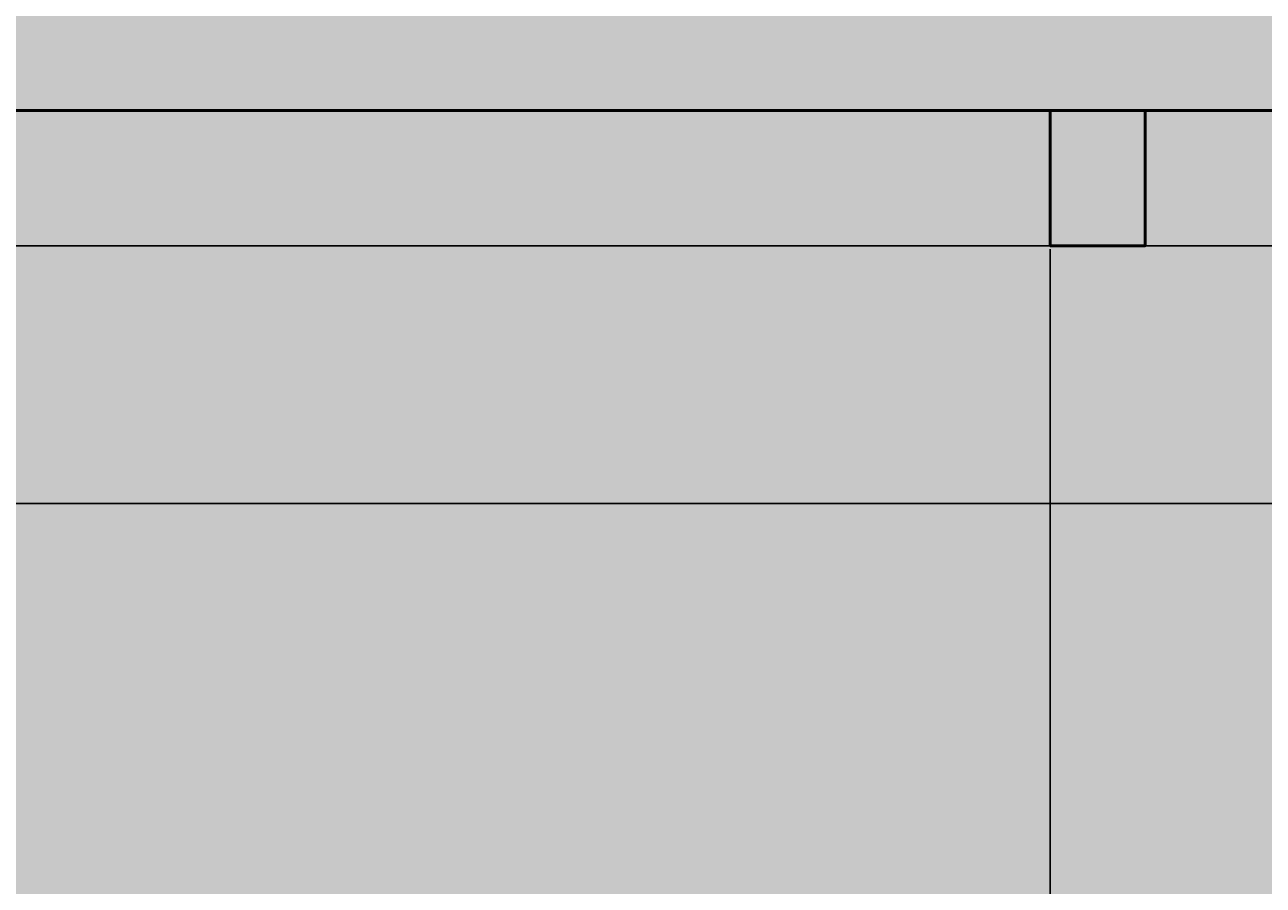
# Model space of a CAD drawing. Units: inches. Extents: x -12 to 334, y -10 to 186.
# Tile 41 of 77: x 152 to 175, y 49 to 65. Entities that reach past the tile are written whole.
import ezdxf

# ---------------------------------------------------------------- set-up
doc = ezdxf.new("R2010")
doc.units = ezdxf.units.IN
doc.header["$MEASUREMENT"] = 0
for name, color, linetype, lineweight in [('M-DIMS', 2, 'Continuous', 18), ('M-EQPM', 7, 'Continuous', 50), ('M-EQPM-PATT', 8, 'Continuous', 18)]:
    doc.layers.add(name, color=color, linetype=linetype, lineweight=lineweight)
doc.styles.get("Standard").update_dxf_attribs({"font": 'arial.ttf'})
doc.dimstyles.get("Standard").update_dxf_attribs({"dimtxt": 0.18, "dimasz": 0.18, "dimexe": 0.18, "dimexo": 0.0625, "dimgap": 0.09, "dimtad": 0, "dimtih": 1, "dimtoh": 1, "dimdec": 4, "dimzin": 0, "dimdsep": 46, "dimtxsty": 'Standard', "dimcen": 0.09, "dimadec": 0, "dimazin": 0, "dimtfac": 1, "dimtdec": 4, "dimtofl": 0, "dimtmove": 0, "dimatfit": 3, "dimfxl": 1, "dimtolj": 1, "dimtzin": 0, "dimarcsym": 0})

# ---------------------------------------------------------------- blocks, each defined once
blk = doc.blocks.new('*D1')
at = {"layer": 'Defpoints', "color": 0, "transparency": 16777216}
for p in [(281.426, 91.899), (3.376, 80.692), (281.426, 14.304)]:
    blk.add_point(p, dxfattribs=at)
at = {"layer": 'M-DIMS', "color": 0, "lineweight": -2, "transparency": 16777216}
for p, q in [((281.426, 91.836), (281.426, 14.124)), ((3.376, 80.629), (3.376, 14.124)), ((3.556, 14.304), (141.935, 14.304)), ((281.246, 14.304), (142.867, 14.304))]:
    blk.add_line(p, q, dxfattribs=at)
at = {"layer": 'M-DIMS', "color": 0, "transparency": 16777216}
for points in [[(3.556, 14.334), (3.556, 14.274), (3.376, 14.304)], [(281.246, 14.334), (281.246, 14.274), (281.426, 14.304)]]:
    blk.add_solid(points, dxfattribs=at)
at = {"layer": 'M-DIMS', "color": 0, "transparency": 16777216, "insert": (142.401, 14.304), "char_height": 0.18, "attachment_point": 5}
blk.add_mtext('\\A1;278.05', dxfattribs=at)
blk = doc.blocks.new('*D17')
at = {"layer": 'Defpoints', "color": 0, "transparency": 16777216}
for p in [(106.177, 102.896), (105.892, 56.321), (295.976, 56.321)]:
    blk.add_point(p, dxfattribs=at)
at = {"layer": 'M-DIMS', "color": 0, "lineweight": -2, "transparency": 16777216}
for p, q in [((106.24, 102.896), (296.156, 102.896)), ((295.976, 102.716), (295.976, 79.79)), ((295.976, 56.501), (295.976, 79.426)), ((105.954, 56.321), (296.156, 56.321))]:
    blk.add_line(p, q, dxfattribs=at)
at = {"layer": 'M-DIMS', "color": 0, "transparency": 16777216}
for points in [[(295.946, 102.716), (296.006, 102.716), (295.976, 102.896)], [(295.946, 56.501), (296.006, 56.501), (295.976, 56.321)]]:
    blk.add_solid(points, dxfattribs=at)
at = {"layer": 'M-DIMS', "color": 0, "transparency": 16777216, "insert": (295.976, 79.608), "char_height": 0.18, "attachment_point": 5}
blk.add_mtext('\\A1;46.575', dxfattribs=at)
blk = doc.blocks.new('*D31')
at = {"layer": 'Defpoints', "color": 0, "transparency": 16777216}
for p in [(129.093, 61.105), (170.908, 61.105), (170.908, 14.304)]:
    blk.add_point(p, dxfattribs=at)
at = {"layer": 'M-DIMS', "color": 0, "lineweight": -2, "transparency": 16777216}
for p, q in [((129.093, 61.042), (129.093, 14.124)), ((170.908, 61.042), (170.908, 14.124)), ((129.273, 14.304), (149.532, 14.304)), ((170.728, 14.304), (150.468, 14.304))]:
    blk.add_line(p, q, dxfattribs=at)
at = {"layer": 'M-DIMS', "color": 0, "transparency": 16777216}
for points in [[(129.273, 14.334), (129.273, 14.274), (129.093, 14.304)], [(170.728, 14.334), (170.728, 14.274), (170.908, 14.304)]]:
    blk.add_solid(points, dxfattribs=at)
at = {"layer": 'M-DIMS', "color": 0, "transparency": 16777216, "insert": (150, 14.304), "char_height": 0.18, "attachment_point": 5}
blk.add_mtext('\\A1;41.815', dxfattribs=at)
blk = doc.blocks.new('*D32')
at = {"layer": 'Defpoints', "color": 0, "transparency": 16777216}
for p in [(170.908, 61.105), (216.428, 61.105), (216.428, 14.304)]:
    blk.add_point(p, dxfattribs=at)
at = {"layer": 'M-DIMS', "color": 0, "lineweight": -2, "transparency": 16777216}
for p, q in [((170.908, 61.042), (170.908, 14.124)), ((216.428, 61.042), (216.428, 14.124)), ((171.088, 14.304), (193.271, 14.304)), ((216.248, 14.304), (194.064, 14.304))]:
    blk.add_line(p, q, dxfattribs=at)
at = {"layer": 'M-DIMS', "color": 0, "transparency": 16777216}
for points in [[(171.088, 14.334), (171.088, 14.274), (170.908, 14.304)], [(216.248, 14.334), (216.248, 14.274), (216.428, 14.304)]]:
    blk.add_solid(points, dxfattribs=at)
at = {"layer": 'M-DIMS', "color": 0, "transparency": 16777216, "insert": (193.668, 14.304), "char_height": 0.18, "attachment_point": 5}
blk.add_mtext('\\A1;45.52', dxfattribs=at)
blk = doc.blocks.new('*D35')
at = {"layer": 'Defpoints', "color": 0, "transparency": 16777216}
for p in [(216.428, 98.108), (-11.174, 61.105), (216.428, 61.105)]:
    blk.add_point(p, dxfattribs=at)
at = {"layer": 'M-DIMS', "color": 0, "lineweight": -2, "transparency": 16777216}
for p, q in [((216.365, 98.108), (-11.354, 98.108)), ((-11.174, 97.928), (-11.174, 79.788)), ((-11.174, 61.285), (-11.174, 79.424)), ((216.365, 61.105), (-11.354, 61.105))]:
    blk.add_line(p, q, dxfattribs=at)
at = {"layer": 'M-DIMS', "color": 0, "transparency": 16777216}
for points in [[(-11.204, 97.928), (-11.144, 97.928), (-11.174, 98.108)], [(-11.204, 61.285), (-11.144, 61.285), (-11.174, 61.105)]]:
    blk.add_solid(points, dxfattribs=at)
at = {"layer": 'M-DIMS', "color": 0, "transparency": 16777216, "insert": (-11.174, 79.606), "char_height": 0.18, "attachment_point": 5}
blk.add_mtext('\\A1;37', dxfattribs=at)
blk = doc.blocks.new('*D39')
at = {"layer": 'Defpoints', "color": 0, "transparency": 16777216}
for p in [(279.726, 80.692), (-11.174, 45.854), (269.381, 45.854)]:
    blk.add_point(p, dxfattribs=at)
at = {"layer": 'M-DIMS', "color": 0, "lineweight": -2, "transparency": 16777216}
for p, q in [((279.664, 80.692), (-11.354, 80.692)), ((-11.174, 80.512), (-11.174, 63.455)), ((-11.174, 46.034), (-11.174, 63.091)), ((269.318, 45.854), (-11.354, 45.854))]:
    blk.add_line(p, q, dxfattribs=at)
at = {"layer": 'M-DIMS', "color": 0, "transparency": 16777216}
for points in [[(-11.204, 80.512), (-11.144, 80.512), (-11.174, 80.692)], [(-11.204, 46.034), (-11.144, 46.034), (-11.174, 45.854)]]:
    blk.add_solid(points, dxfattribs=at)
at = {"layer": 'M-DIMS', "color": 0, "transparency": 16777216, "insert": (-11.174, 63.273), "char_height": 0.18, "attachment_point": 5}
blk.add_mtext('\\A1;34.84', dxfattribs=at)

msp = doc.modelspace()

# ---------------------------------------------------------------- hatches: boundary and pattern name
at = {"layer": 'M-EQPM-PATT'}
h = msp.add_hatch(color=256, dxfattribs=at)
h.set_gradient(color1=(205, 32, 39), color2=(205, 32, 39), tint=1)
h.paths.add_polyline_path([(64.5, 80.754), (64.5, 89.8963), (226.6083, 89.8963, -1), (226.6083, 69.6117), (64.5, 69.6117), (64.5, 78.754), (4.4744, 78.754, 0.384914), (23.5807, 61.4872), (37.1002, 61.4872), (37.1002, 33.6752), (53.1002, 33.6752), (53.1002, 61.4872), (64.5, 61.4872), (64.5, 63.6117), (226.6083, 63.6117, 1), (226.6083, 95.8963), (64.5, 95.8963), (64.5, 99.8958), (53.1002, 99.8958), (53.1002, 127.7078), (37.1002, 127.7078), (37.1002, 99.8958), (23.5807, 99.8958, 0.4132606), (4.3766, 80.754)])
h.paths.add_polyline_path([(64.5, 91.8963), (64.5, 93.8963), (226.6083, 93.8963, -1), (226.6083, 65.6117), (64.5, 65.6117), (64.5, 67.6117), (226.6083, 67.6117, 1), (226.6083, 91.8963)], flags=16)
h = msp.add_hatch(color=256, dxfattribs=at)
h.set_gradient(color1=(99, 100, 102), color2=(99, 100, 102), tint=1)
h.paths.add_polyline_path([(72.9244, 95.8963), (75.9244, 95.8963), (75.9244, 109.0583), (72.9244, 109.0583)])
h.paths.add_polyline_path([(72.9244, 50.4497), (75.9244, 50.4497), (75.9244, 63.6117), (72.9244, 63.6117)])
h.paths.add_polyline_path([(75.9244, 91.8963), (75.9244, 93.8963), (72.9244, 93.8963), (72.9244, 91.8963)])
h.paths.add_polyline_path([(75.9244, 65.6117), (75.9244, 67.6117), (72.9244, 67.6117), (72.9244, 65.6117)])
h.paths.add_polyline_path([(129.093, 69.6117), (130.8573, 69.6117), (130.8573, 89.8963), (129.093, 89.8963)])
h.paths.add_polyline_path([(129.093, 98.1081), (129.093, 95.8963), (130.8573, 95.8963), (130.8573, 98.1081)])
h.paths.add_polyline_path([(130.8573, 61.1045), (130.8573, 63.6117), (129.093, 63.6117), (129.093, 61.1045)])
h.paths.add_polyline_path([(170.9079, 69.6117), (172.6722, 69.6117), (172.6722, 89.8963), (170.9079, 89.8963)])
h.paths.add_polyline_path([(172.6722, 95.8963), (172.6722, 98.1081), (170.9079, 98.1081), (170.9079, 95.8963)])
h.paths.add_polyline_path([(170.9079, 61.1045), (172.6722, 61.1045), (172.6722, 63.6117), (170.9079, 63.6117)])
h.paths.add_polyline_path([(218.1922, 63.6117), (216.4278, 63.6117), (216.4278, 61.1045), (218.1922, 61.1045)])
h.paths.add_polyline_path([(216.4278, 69.6117), (218.1922, 69.6117), (218.1922, 89.8963), (216.4278, 89.8963)])
h.paths.add_polyline_path([(216.4278, 95.8963), (218.1922, 95.8963), (218.1922, 98.1081), (216.4278, 98.1081)])
h = msp.add_hatch(color=256, dxfattribs=at)
h.set_gradient(color1=(94, 103, 175), color2=(94, 103, 175), tint=1)
h.paths.add_polyline_path([(129.093, 89.8963), (86.8879, 89.8963), (86.8879, 69.6117), (129.093, 69.6117)], flags=17)
h.paths.add_polyline_path([(170.9079, 89.8963), (130.8573, 89.8963), (130.8573, 69.6117), (170.9079, 69.6117)], flags=17)
h.paths.add_polyline_path([(216.4278, 89.8963), (172.6722, 89.8963), (172.6722, 69.6117), (216.4278, 69.6117)], flags=17)
h.paths.add_polyline_path([(245.9354, 82.6969), (247.9354, 82.6969), (247.9354, 46.8541), (268.3808, 46.8541, 0.0998398), (279.7263, 80.6915), (251.9801, 80.6915, 0.4142136), (231.7758, 100.8958), (84.7229, 100.8958), (84.7229, 109.0583), (83.7229, 109.0583), (83.7229, 95.8963), (129.093, 95.8963), (129.093, 98.1081), (130.8573, 98.1081), (130.8573, 95.8963), (170.9079, 95.8963), (170.9079, 98.1081), (172.6722, 98.1081), (172.6722, 95.8963), (216.4278, 95.8963), (216.4278, 98.1081), (218.1922, 98.1081), (218.1922, 95.8963), (226.6083, 95.8963, -1), (226.6083, 63.6117), (218.1922, 63.6117), (218.1922, 61.1045), (216.4278, 61.1045), (216.4278, 63.6117), (172.6722, 63.6117), (172.6722, 61.1045), (170.9079, 61.1045), (170.9079, 63.6117), (130.8573, 63.6117), (130.8573, 61.1045), (129.093, 61.1045), (129.093, 63.6117), (87.8879, 63.6117), (87.8879, 56.3205), (105.8919, 56.3205), (105.8919, 28.8541), (115.8919, 28.8541), (115.8919, 46.8541), (222.5761, 46.8541), (222.5761, 30.8541), (232.5761, 30.8541), (232.5761, 46.8541), (245.9354, 46.8541)])
h.paths.add_polyline_path([(86.8879, 89.8963), (75.9244, 89.8963), (75.9244, 69.6117), (86.8879, 69.6117)])
h.paths.add_polyline_path([(83.7229, 109.0583), (75.9244, 109.0583), (75.9244, 95.8963), (83.7229, 95.8963)])
h.paths.add_polyline_path([(226.6083, 89.8963), (218.1922, 89.8963), (218.1922, 69.6117), (226.6083, 69.6117, 1)], flags=17)
h = msp.add_hatch(color=256, dxfattribs=at)
h.set_gradient(color1=(0, 0, 255), color2=(0, 0, 255), tint=1)
h.paths.add_polyline_path([(84.7229, 100.8958), (84.7229, 109.0583), (83.7229, 109.0583), (83.7229, 95.8963), (129.093, 95.8963), (129.093, 98.1081), (130.8573, 98.1081), (130.8573, 95.8963), (170.9079, 95.8963), (170.9079, 98.1081), (172.6722, 98.1081), (172.6722, 95.8963), (216.4278, 95.8963), (216.4278, 98.1081), (218.1922, 98.1081), (218.1922, 95.8963), (226.6083, 95.8963, -1), (226.6083, 63.6117), (218.1922, 63.6117), (218.1922, 61.1045), (216.4278, 61.1045), (216.4278, 63.6117), (172.6722, 63.6117), (172.6722, 61.1045), (170.9079, 61.1045), (170.9079, 63.6117), (130.8573, 63.6117), (130.8573, 61.1045), (129.093, 61.1045), (129.093, 63.6117), (87.8879, 63.6117), (87.8879, 56.3205), (105.8919, 56.3205), (105.8919, 28.8541), (115.8919, 28.8541), (115.8919, 46.8541), (222.5761, 46.8541), (222.5761, 30.8541), (232.5761, 30.8541), (232.5761, 46.8541), (245.9354, 46.8541), (245.9354, 82.6969), (247.9354, 82.6969), (247.9354, 46.8541), (268.3808, 46.8541, 0.0998398), (279.7263, 80.6915), (251.9801, 80.6915, 0.4142136), (231.7758, 100.8958)])

# ---------------------------------------------------------------- linework, layer by layer
at = {"layer": 'M-EQPM'}
msp.add_lwpolyline([(64.5, 63.6117), (226.6083, 63.6117, 1), (226.6083, 95.8963), (64.5, 95.8963)], format="xyb", dxfattribs=at)
msp.add_lwpolyline([(172.6722, 63.6117), (172.6722, 61.1045), (170.9079, 61.1045), (170.9079, 63.6117)], dxfattribs=at)

# ---------------------------------------------------------------- dimensions: what is measured, and where the dimension line sits
at = {"layer": 'M-DIMS'}
for base, p1, p2, override, picture, middle in [((295.9756, 56.3205), (106.1771, 102.8958), (105.8919, 56.3205), {"dimdec": 3, "dimlfac": 1, "dimrnd": 0, "dimzin": 0, "dimdsep": 46, "dimlunit": 2}, '*D17', (295.9756, 79.6082)), ((-11.1736, 61.1045), (216.4278, 98.1081), (216.4278, 61.1045), {"dimdec": 0, "dimlfac": 1, "dimrnd": 0, "dimzin": 0, "dimdsep": 46, "dimlunit": 2}, '*D35', (-11.1735, 79.6063)), ((-11.1736, 45.8541), (279.7263, 80.6915), (269.3808, 45.8541), {"dimdec": 2, "dimlfac": 1, "dimrnd": 0, "dimzin": 0, "dimdsep": 46, "dimlunit": 2}, '*D39', (-11.1735, 63.2728))]:
    dim = msp.add_linear_dim(base=base, p1=p1, p2=p2, angle=90, dimstyle='Standard', override=override, dxfattribs=at)
    dim.commit()
    dim.dimension.update_dxf_attribs({"geometry": picture, "text_midpoint": middle})
for base, p1, p2, override, picture, middle in [((281.4256, 14.3041), (3.3765, 80.6915), (281.4256, 91.8988), {"dimdec": 2, "dimlfac": 1, "dimrnd": 0, "dimzin": 0, "dimdsep": 46, "dimlunit": 2}, '*D1', (142.401, 14.3041)), ((170.9079, 14.3041), (129.093, 61.1045), (170.9079, 61.1045), {"dimdec": 3, "dimlfac": 1, "dimrnd": 0, "dimzin": 0, "dimdsep": 46, "dimlunit": 2}, '*D31', (150.0004, 14.3041)), ((216.4278, 14.3041), (170.9079, 61.1045), (216.4278, 61.1045), {"dimdec": 2, "dimlfac": 1, "dimrnd": 0, "dimzin": 0, "dimdsep": 46, "dimlunit": 2}, '*D32', (193.6678, 14.3041))]:
    dim = msp.add_linear_dim(base=base, p1=p1, p2=p2, dimstyle='Standard', override=override, dxfattribs=at)
    dim.commit()
    dim.dimension.update_dxf_attribs({"geometry": picture, "text_midpoint": middle})

doc.saveas('drawing.dxf')
